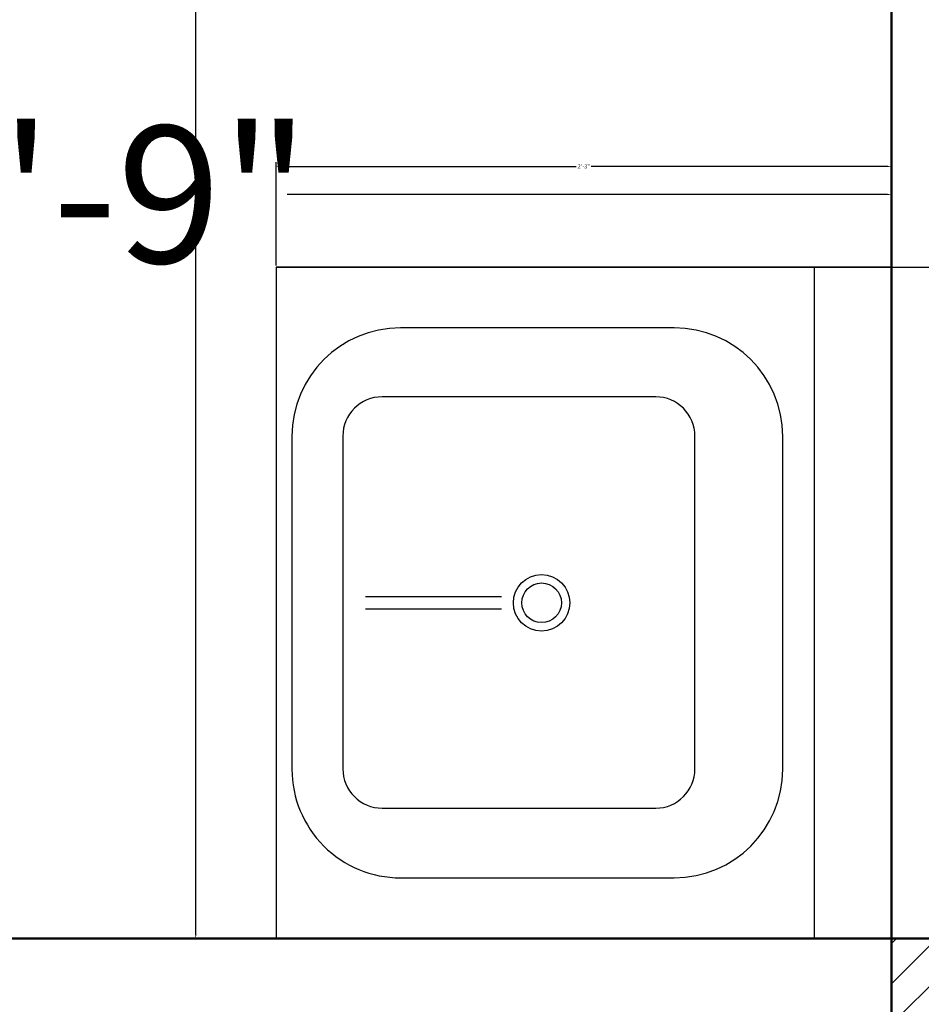
# Model space of a CAD drawing. Units: inches. Extents: x 0 to 281, y -535 to 46.
# Tile 12 of 22: x 196 to 236, y -125 to -82. Entities that reach past the tile are written whole.
import ezdxf

# ---------------------------------------------------------------- set-up
doc = ezdxf.new("R2010")
doc.units = ezdxf.units.IN
doc.header["$MEASUREMENT"] = 0
for name, color, linetype, lineweight in [('A-ANNO-DIMS', 2, 'Continuous', 18), ('A-COLS-PATT', 152, 'Continuous', 13), ('A-FLOR-FIXT', 9, 'Continuous', 25), ('A-WALL', 7, 'Continuous', 50)]:
    doc.layers.add(name, color=color, linetype=linetype, lineweight=lineweight)
doc.styles.get("Standard").update_dxf_attribs({"font": 'arial.ttf'})
doc.dimstyles.get("Standard").update_dxf_attribs({"dimtxt": 0.18, "dimasz": 0.18, "dimexe": 0.18, "dimexo": 0.0625, "dimgap": 0.09, "dimtad": 0, "dimtih": 1, "dimtoh": 1, "dimdec": 0, "dimzin": 0, "dimdsep": 46, "dimlunit": 3, "dimtxsty": 'Standard', "dimcen": 0.09, "dimadec": 0, "dimazin": 0, "dimtfac": 1, "dimtdec": 0, "dimtofl": 0, "dimtmove": 0, "dimatfit": 3, "dimfxl": 1, "dimtolj": 1, "dimtzin": 0, "dimarcsym": 0})

# ---------------------------------------------------------------- blocks, each defined once
blk = doc.blocks.new('*D3')
at = {"layer": 'A-ANNO-DIMS', "color": 0, "lineweight": -2, "transparency": 16777216}
for p, q in [((204.079, 9.589), (204.197, 9.589)), ((204.017, 9.409), (204.017, -53.308)), ((204.017, -122.231), (204.017, -59.513)), ((204.079, -122.411), (204.197, -122.411))]:
    blk.add_line(p, q, dxfattribs=at)
at = {"layer": 'A-ANNO-DIMS', "color": 0, "transparency": 16777216}
for points in [[(203.987, 9.409), (204.047, 9.409), (204.017, 9.589)], [(203.987, -122.231), (204.047, -122.231), (204.017, -122.411)]]:
    blk.add_solid(points, dxfattribs=at)
at = {"layer": 'Defpoints', "color": 0, "transparency": 16777216}
for p in [(204.017, 9.589), (204.017, -122.411), (204.017, -122.411)]:
    blk.add_point(p, dxfattribs=at)
at = {"layer": 'A-ANNO-DIMS', "color": 0, "transparency": 16777216, "insert": (204.017, -56.411), "char_height": 6, "attachment_point": 5}
blk.add_mtext("\\A1;11'", dxfattribs=at)
blk = doc.blocks.new('*D4')
at = {"layer": 'A-ANNO-DIMS', "color": 0, "lineweight": -2, "transparency": 16777216}
for p, q in [((165.459, -89.775), (165.459, -89.658)), ((234.459, -89.775), (234.459, -89.658)), ((165.639, -89.838), (191.894, -89.838)), ((234.279, -89.838), (208.024, -89.838))]:
    blk.add_line(p, q, dxfattribs=at)
at = {"layer": 'A-ANNO-DIMS', "color": 0, "transparency": 16777216}
for points in [[(165.639, -89.808), (165.639, -89.868), (165.459, -89.838)], [(234.279, -89.808), (234.279, -89.868), (234.459, -89.838)]]:
    blk.add_solid(points, dxfattribs=at)
at = {"layer": 'Defpoints', "color": 0, "transparency": 16777216}
for p in [(165.459, -89.838), (234.459, -89.838), (234.459, -89.838)]:
    blk.add_point(p, dxfattribs=at)
at = {"layer": 'A-ANNO-DIMS', "color": 0, "transparency": 16777216, "insert": (199.959, -89.838), "char_height": 6, "attachment_point": 5}
blk.add_mtext('\\A1;5\'-9"', dxfattribs=at)
blk = doc.blocks.new('М14 600х655')
for p, q in [((-655, 600), (-655, 0)), ((-655, 600), (-655, 0)), ((-655, 0), (-655, 600)), ((0, 600), (-655, 600)), ((0, 0), (0, 600)), ((0, 525), (-655, 525)), ((-165.12, 494.05), (-489.88, 494.05)), ((-165.43, 408.39), (-490.19, 408.39)), ((-595.78, 388.15), (-595.78, 121.32)), ((-59.22, 121.32), (-59.22, 388.15)), ((-528.43, 370.14), (-528.43, 103.31)), ((-127.19, 103.31), (-127.19, 370.14)), ((-333.51, 87.11), (-333.51, 219.65)), ((-321.49, 87.11), (-321.49, 219.65)), ((-490.19, 65.07), (-165.43, 65.07)), ((-489.88, 15.41), (-165.12, 15.41)), ((-655, 0), (-655, 0)), ((-655, 0), (-655, 0)), ((-655, 0), (0, 0)), ((-655, 0), (0, 0))]:
    blk.add_line(p, q)
for radius in [27.55, 19.33]:
    blk.add_circle((-327.5, 258.9), radius)
for centre, radius, start, end in [((-489.88, 388.15), 105.9, 90, 180), ((-165.12, 388.15), 105.9, 0, 90), ((-490.19, 370.14), 38.24, 90, 180), ((-165.43, 370.14), 38.24, 0, 90), ((-489.88, 121.32), 105.9, 180, 270), ((-165.12, 121.32), 105.9, 270, 0), ((-490.19, 103.31), 38.24, 180, 270), ((-165.43, 103.31), 38.24, 270, 0)]:
    blk.add_arc(centre, radius, start, end)
blk = doc.blocks.new('*D30')
at = {"layer": 'A-ANNO-DIMS', "color": 0, "lineweight": -2, "transparency": 16777216}
for p, q in [((234.521, -93.018), (239.048, -93.018)), ((238.868, -93.198), (238.868, -107.531)), ((238.868, -122.231), (238.868, -107.897)), ((234.521, -122.411), (239.048, -122.411))]:
    blk.add_line(p, q, dxfattribs=at)
at = {"layer": 'A-ANNO-DIMS', "color": 0, "transparency": 16777216}
for points in [[(238.838, -93.198), (238.898, -93.198), (238.868, -93.018)], [(238.838, -122.231), (238.898, -122.231), (238.868, -122.411)]]:
    blk.add_solid(points, dxfattribs=at)
at = {"layer": 'Defpoints', "color": 0, "transparency": 16777216}
for p in [(234.459, -93.018), (234.459, -122.411), (238.868, -122.411)]:
    blk.add_point(p, dxfattribs=at)
at = {"layer": 'A-ANNO-DIMS', "color": 0, "transparency": 16777216, "insert": (238.868, -107.714), "char_height": 0.18, "attachment_point": 5}
blk.add_mtext('\\A1;KITCHEN SINK 2\'-5 1/2"', dxfattribs=at)
blk = doc.blocks.new('*D31')
at = {"layer": 'A-ANNO-DIMS', "color": 0, "lineweight": -2, "transparency": 16777216}
for p, q in [((207.534, -92.955), (207.534, -88.429)), ((207.714, -88.609), (220.666, -88.609)), ((234.279, -88.609), (221.327, -88.609)), ((234.459, -92.955), (234.459, -88.429))]:
    blk.add_line(p, q, dxfattribs=at)
at = {"layer": 'A-ANNO-DIMS', "color": 0, "transparency": 16777216}
for points in [[(207.714, -88.579), (207.714, -88.639), (207.534, -88.609)], [(234.279, -88.579), (234.279, -88.639), (234.459, -88.609)]]:
    blk.add_solid(points, dxfattribs=at)
at = {"layer": 'Defpoints', "color": 0, "transparency": 16777216}
for p in [(234.459, -88.609), (207.534, -93.018), (234.459, -93.018)]:
    blk.add_point(p, dxfattribs=at)
at = {"layer": 'A-ANNO-DIMS', "color": 0, "transparency": 16777216, "insert": (220.997, -88.609), "char_height": 0.18, "attachment_point": 5}
blk.add_mtext('\\A1;2\'-3"', dxfattribs=at)

msp = doc.modelspace()

# ---------------------------------------------------------------- hatches: boundary and pattern name
at = {"layer": 'A-COLS-PATT'}
h = msp.add_hatch(dxfattribs=at)
h.set_pattern_fill('ANSI31', color=256, scale=10)
h.paths.add_polyline_path([(36.459, 18.589), (27.459, 18.589), (27.459, 9.589), (36.459, 9.589)])
h.paths.add_polyline_path([(165.459, 18.589), (156.459, 18.589), (156.459, 9.589), (165.459, 9.589)])
h.paths.add_polyline_path([(243.459, 18.589), (234.459, 18.589), (234.459, 9.589), (243.459, 9.589)])
h.paths.add_polyline_path([(243.459, -122.411), (234.459, -122.411), (234.459, -131.411), (243.459, -131.411)])
h.paths.add_polyline_path([(36.459, -122.411), (27.459, -122.411), (27.459, -131.411), (36.459, -131.411)])
h.paths.add_polyline_path([(36.459, -498.411), (27.459, -498.411), (27.459, -507.411), (36.459, -507.411)])
h.paths.add_polyline_path([(243.459, -498.411), (234.459, -498.411), (234.459, -507.411), (243.459, -507.411)])
h.paths.add_polyline_path([(159.459, -498.411), (150.459, -498.411), (150.459, -507.411), (159.459, -507.411)])
h.paths.add_polyline_path([(36.459, -392.411), (27.459, -392.411), (27.459, -401.411), (36.459, -401.411)])
h.paths.add_polyline_path([(159.459, -392.411), (150.459, -392.411), (150.459, -401.411), (159.459, -401.411)])
h.paths.add_polyline_path([(243.459, -392.411), (234.459, -392.411), (234.459, -401.411), (243.459, -401.411)])
h.paths.add_polyline_path([(36.459, -263.411), (27.459, -263.411), (27.459, -272.411), (36.459, -272.411)])
h.paths.add_polyline_path([(243.459, -263.411), (234.459, -263.411), (234.459, -272.411), (243.459, -272.411)])

# ---------------------------------------------------------------- linework, layer by layer
at = {"layer": 'A-WALL'}
for p, q in [((234.459, 18.589), (234.459, -507.411)), ((189.459, -122.411), (243.459, -122.411))]:
    msp.add_line(p, q, dxfattribs=at)

# ---------------------------------------------------------------- block references
at = {"layer": 'A-FLOR-FIXT', "xscale": 0.0448741256333582, "yscale": 0.0448741256333582, "zscale": 0.0448741256333582, "rotation": 270}
msp.add_blockref('М14 600х655', (207.534, -122.411), dxfattribs=at)

# ---------------------------------------------------------------- dimensions: what is measured, and where the dimension line sits
at = {"layer": 'A-ANNO-DIMS'}
dim = msp.add_linear_dim(base=(204.017, -122.411), p1=(204.017, 9.589), p2=(204.017, -122.411), angle=90, dimstyle='Standard', override={"dimtxt": 6, "dimclrd": 0, "dimclre": 0, "dimclrt": 0}, dxfattribs=at)
dim.commit()
dim.dimension.update_dxf_attribs({"geometry": '*D3', "text_midpoint": (204.017, -56.411)})
for base, p1, p2, override, picture, middle in [((234.459, -89.838), (165.459, -89.838), (234.459, -89.838), {"dimtxt": 6, "dimclrd": 0, "dimclre": 0, "dimclrt": 0}, '*D4', (199.959, -89.838)), ((234.459, -88.609), (207.534, -93.018), (234.459, -93.018), {"dimdec": 1, "dimlfac": 1, "dimrnd": 0, "dimzin": 1, "dimdsep": 46, "dimlunit": 4, "dimfrac": 2}, '*D31', (220.997, -88.609))]:
    dim = msp.add_linear_dim(base=base, p1=p1, p2=p2, dimstyle='Standard', override=override, dxfattribs=at)
    dim.commit()
    dim.dimension.update_dxf_attribs({"geometry": picture, "text_midpoint": middle})
dim = msp.add_linear_dim(base=(238.868, -122.411), p1=(234.459, -93.018), p2=(234.459, -122.411), angle=270, text='KITCHEN SINK <>', dimstyle='Standard', override={"dimdec": 1, "dimlfac": 1, "dimrnd": 0, "dimzin": 1, "dimdsep": 46, "dimlunit": 4, "dimfrac": 2}, dxfattribs=at)
dim.commit()
dim.dimension.update_dxf_attribs({"geometry": '*D30', "text_midpoint": (238.868, -107.714)})

doc.saveas('drawing.dxf')
